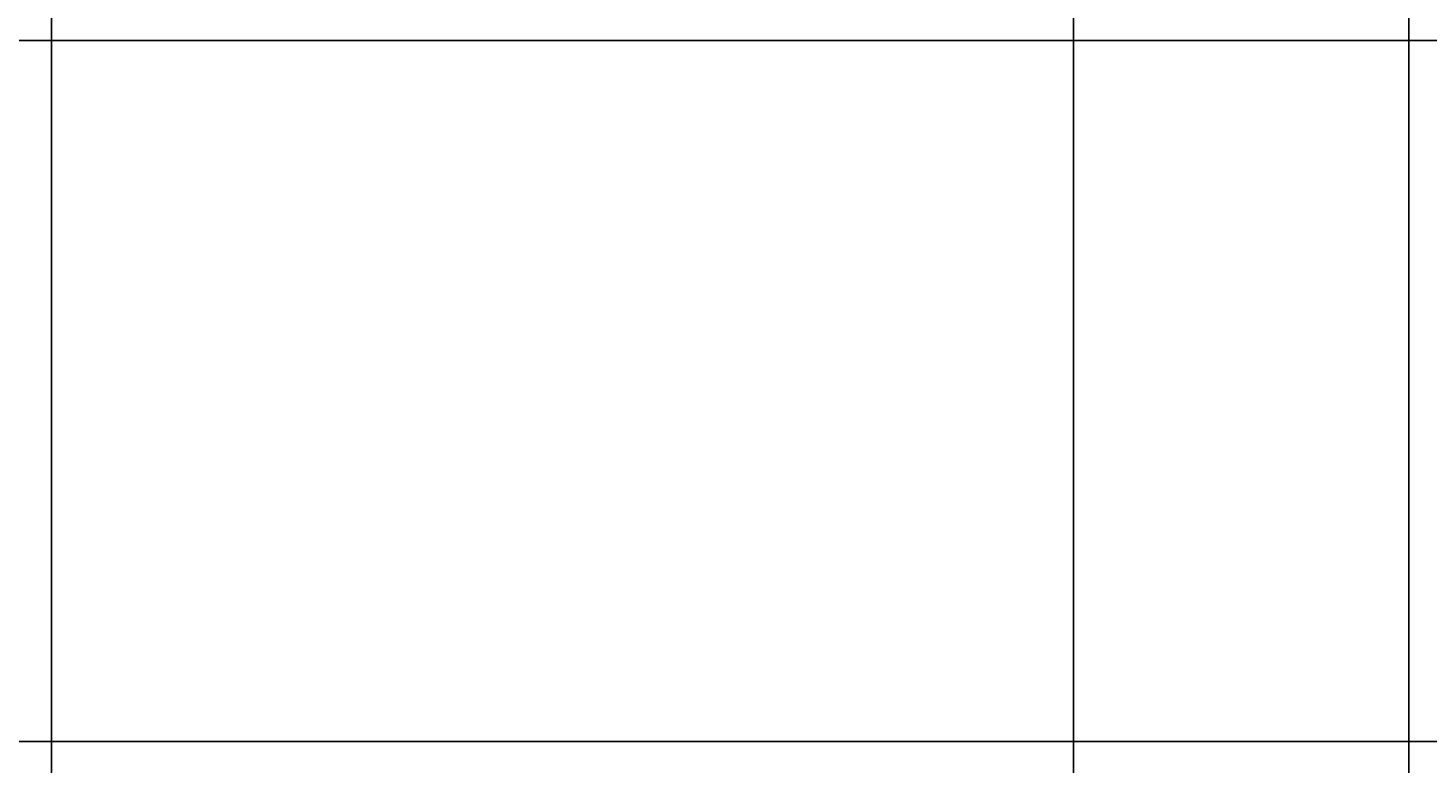
# Model space of a CAD drawing. Units: inches. Extents: x 35362 to 73946, y 43607 to 67532.
# Tile 84 of 134: x 50119 to 51337, y 47689 to 48329. Entities that reach past the tile are written whole.
import ezdxf

# ---------------------------------------------------------------- set-up
doc = ezdxf.new("R2010")
doc.units = ezdxf.units.IN
doc.header["$MEASUREMENT"] = 0
doc.layers.add('A-ANNO-DIMS', color=2, linetype='Continuous', lineweight=18)
doc.styles.get("Standard").update_dxf_attribs({"font": 'arial.ttf'})
doc.dimstyles.get("Standard").update_dxf_attribs({"dimtxt": 0.18, "dimasz": 0.18, "dimexe": 0.18, "dimexo": 0.0625, "dimgap": 0.09, "dimtad": 0, "dimtih": 1, "dimtoh": 1, "dimdec": 4, "dimzin": 0, "dimdsep": 46, "dimtxsty": 'Standard', "dimcen": 0.09, "dimadec": 0, "dimazin": 0, "dimtfac": 1, "dimtdec": 4, "dimtofl": 0, "dimtmove": 0, "dimatfit": 3, "dimfxl": 1, "dimtolj": 1, "dimtzin": 0, "dimarcsym": 0})

# ---------------------------------------------------------------- blocks, each defined once
blk = doc.blocks.new('*D11')
at = {"layer": 'A-ANNO-DIMS', "color": 0, "lineweight": -2, "transparency": 16777216}
for p, q in [((47978.7, 56028.8), (47978.7, 43606.7)), ((53109.8, 56028.8), (53109.8, 43606.7)), ((47978.8, 43606.9), (50543.9, 43606.9)), ((53109.6, 43606.9), (50544.6, 43606.9))]:
    blk.add_line(p, q, dxfattribs=at)
at = {"layer": 'A-ANNO-DIMS', "color": 0, "transparency": 16777216}
for points in [[(47978.8, 43606.9), (47978.8, 43606.8), (47978.7, 43606.9)], [(53109.6, 43606.9), (53109.6, 43606.8), (53109.8, 43606.9)]]:
    blk.add_solid(points, dxfattribs=at)
at = {"layer": 'Defpoints', "color": 0, "transparency": 16777216}
for p in [(47978.7, 56028.8), (53109.8, 56028.8), (53109.8, 43606.9)]:
    blk.add_point(p, dxfattribs=at)
at = {"layer": 'A-ANNO-DIMS', "color": 0, "transparency": 16777216, "insert": (50544.2, 43606.9), "char_height": 0.18, "attachment_point": 5}
blk.add_mtext('\\A1;5131', dxfattribs=at)
blk = doc.blocks.new('*D13')
at = {"layer": 'A-ANNO-DIMS', "color": 0, "lineweight": -2, "transparency": 16777216}
for p, q in [((48373.5, 51694), (48373.5, 43606.7)), ((51029, 51694), (51029, 43606.7)), ((48373.7, 43606.9), (49700.8, 43606.9)), ((51028.9, 43606.9), (49701.7, 43606.9))]:
    blk.add_line(p, q, dxfattribs=at)
at = {"layer": 'A-ANNO-DIMS', "color": 0, "transparency": 16777216}
for points in [[(48373.7, 43606.9), (48373.7, 43606.8), (48373.5, 43606.9)], [(51028.9, 43606.9), (51028.9, 43606.8), (51029, 43606.9)]]:
    blk.add_solid(points, dxfattribs=at)
at = {"layer": 'Defpoints', "color": 0, "transparency": 16777216}
for p in [(48373.5, 51694.1), (51029, 51694.1), (51029, 43606.9)]:
    blk.add_point(p, dxfattribs=at)
at = {"layer": 'A-ANNO-DIMS', "color": 0, "transparency": 16777216, "insert": (49701.3, 43606.9), "char_height": 0.18, "attachment_point": 5}
blk.add_mtext('\\A1;2655.6', dxfattribs=at)
blk = doc.blocks.new('*D17')
at = {"layer": 'A-ANNO-DIMS', "color": 0, "lineweight": -2, "transparency": 16777216}
for p, q in [((49923.3, 61293.2), (49923.3, 43606.7)), ((51913.9, 61293.2), (51913.9, 43606.7)), ((49923.5, 43606.9), (50918.2, 43606.9)), ((51913.8, 43606.9), (50919.1, 43606.9))]:
    blk.add_line(p, q, dxfattribs=at)
at = {"layer": 'A-ANNO-DIMS', "color": 0, "transparency": 16777216}
for points in [[(49923.5, 43606.9), (49923.5, 43606.8), (49923.3, 43606.9)], [(51913.8, 43606.9), (51913.8, 43606.8), (51913.9, 43606.9)]]:
    blk.add_solid(points, dxfattribs=at)
at = {"layer": 'Defpoints', "color": 0, "transparency": 16777216}
for p in [(49923.3, 61293.3), (51913.9, 61293.3), (51913.9, 43606.9)]:
    blk.add_point(p, dxfattribs=at)
at = {"layer": 'A-ANNO-DIMS', "color": 0, "transparency": 16777216, "insert": (50918.6, 43606.9), "char_height": 0.18, "attachment_point": 5}
blk.add_mtext('\\A1;1990.6', dxfattribs=at)
blk = doc.blocks.new('*D67')
at = {"layer": 'A-ANNO-DIMS', "color": 0, "lineweight": -2, "transparency": 16777216}
for p, q in [((56873.5, 53351.5), (35361.8, 53351.5)), ((35361.9, 53351.3), (35361.9, 49400.9)), ((35361.9, 45450.1), (35361.9, 49400.5)), ((53793.6, 45449.9), (35361.8, 45449.9))]:
    blk.add_line(p, q, dxfattribs=at)
at = {"layer": 'A-ANNO-DIMS', "color": 0, "transparency": 16777216}
for points in [[(35361.9, 53351.3), (35362, 53351.3), (35361.9, 53351.5)], [(35361.9, 45450.1), (35362, 45450.1), (35361.9, 45449.9)]]:
    blk.add_solid(points, dxfattribs=at)
at = {"layer": 'Defpoints', "color": 0, "transparency": 16777216}
for p in [(35361.9, 53351.5), (56873.6, 53351.5), (53793.6, 45449.9)]:
    blk.add_point(p, dxfattribs=at)
at = {"layer": 'A-ANNO-DIMS', "color": 0, "transparency": 16777216, "insert": (35361.9, 49400.7), "char_height": 0.18, "attachment_point": 5}
blk.add_mtext('\\A1;7901.6', dxfattribs=at)
blk = doc.blocks.new('*D87')
at = {"layer": 'A-ANNO-DIMS', "color": 0, "lineweight": -2, "transparency": 16777216}
for p, q in [((52362.5, 48318.3), (35361.8, 48318.3)), ((35361.9, 48318.1), (35361.9, 47931.4)), ((35361.9, 47544.3), (35361.9, 47931)), ((52362.5, 47544.1), (35361.8, 47544.1))]:
    blk.add_line(p, q, dxfattribs=at)
at = {"layer": 'A-ANNO-DIMS', "color": 0, "transparency": 16777216}
for points in [[(35361.9, 48318.1), (35362, 48318.1), (35361.9, 48318.3)], [(35361.9, 47544.3), (35362, 47544.3), (35361.9, 47544.1)]]:
    blk.add_solid(points, dxfattribs=at)
at = {"layer": 'Defpoints', "color": 0, "transparency": 16777216}
for p in [(35361.9, 48318.3), (52362.6, 48318.3), (52362.6, 47544.1)]:
    blk.add_point(p, dxfattribs=at)
at = {"layer": 'A-ANNO-DIMS', "color": 0, "transparency": 16777216, "insert": (35361.9, 47931.2), "char_height": 0.18, "attachment_point": 5}
blk.add_mtext('\\A1;774.1', dxfattribs=at)
blk = doc.blocks.new('*D89')
at = {"layer": 'A-ANNO-DIMS', "color": 0, "lineweight": -2, "transparency": 16777216}
for p, q in [((53707.7, 48897.7), (35361.8, 48897.7)), ((35361.9, 48897.6), (35361.9, 48303.2)), ((35361.9, 47708.4), (35361.9, 48302.8)), ((53707.7, 47708.2), (35361.8, 47708.2))]:
    blk.add_line(p, q, dxfattribs=at)
at = {"layer": 'A-ANNO-DIMS', "color": 0, "transparency": 16777216}
for points in [[(35361.9, 48897.6), (35362, 48897.6), (35361.9, 48897.7)], [(35361.9, 47708.4), (35362, 47708.4), (35361.9, 47708.2)]]:
    blk.add_solid(points, dxfattribs=at)
at = {"layer": 'Defpoints', "color": 0, "transparency": 16777216}
for p in [(53707.8, 48897.7), (35361.9, 47708.2), (53707.8, 47708.2)]:
    blk.add_point(p, dxfattribs=at)
at = {"layer": 'A-ANNO-DIMS', "color": 0, "transparency": 16777216, "insert": (35361.9, 48303), "char_height": 0.18, "attachment_point": 5}
blk.add_mtext('\\A1;1189.5', dxfattribs=at)
blk = doc.blocks.new('*D107')
at = {"layer": 'A-ANNO-DIMS', "color": 0, "lineweight": -2, "transparency": 16777216}
for p, q in [((50139.6, 59850), (50139.6, 43606.7)), ((51320.8, 59850), (51320.8, 43606.7)), ((50139.7, 43606.9), (50729.7, 43606.9)), ((51320.6, 43606.9), (50730.6, 43606.9))]:
    blk.add_line(p, q, dxfattribs=at)
at = {"layer": 'A-ANNO-DIMS', "color": 0, "transparency": 16777216}
for points in [[(50139.7, 43606.9), (50139.7, 43606.8), (50139.6, 43606.9)], [(51320.6, 43606.9), (51320.6, 43606.8), (51320.8, 43606.9)]]:
    blk.add_solid(points, dxfattribs=at)
at = {"layer": 'Defpoints', "color": 0, "transparency": 16777216}
for p in [(50139.6, 59850.1), (51320.8, 59850.1), (51320.8, 43606.9)]:
    blk.add_point(p, dxfattribs=at)
at = {"layer": 'A-ANNO-DIMS', "color": 0, "transparency": 16777216, "insert": (50730.2, 43606.9), "char_height": 0.18, "attachment_point": 5}
blk.add_mtext('\\A1;1181.3', dxfattribs=at)

msp = doc.modelspace()

# ---------------------------------------------------------------- dimensions: what is measured, and where the dimension line sits
at = {"layer": 'A-ANNO-DIMS'}
for base, p1, p2, override, picture, middle in [((51913.931, 43606.859), (49923.307, 61293.286), (51913.931, 61293.286), {"dimdec": 1, "dimlfac": 1, "dimrnd": 0, "dimzin": 0, "dimdsep": 46, "dimlunit": 2}, '*D17', (50918.619, 43606.859)), ((51320.8133, 43606.859), (50139.5627, 59850.0769), (51320.8133, 59850.0769), {"dimdec": 1, "dimlfac": 1, "dimrnd": 0, "dimzin": 0, "dimdsep": 46, "dimlunit": 2}, '*D107', (50730.188, 43606.859)), ((53109.76, 43606.859), (47978.665, 56028.836), (53109.76, 56028.836), {"dimdec": 0, "dimlfac": 1, "dimrnd": 0, "dimzin": 0, "dimdsep": 46, "dimlunit": 2}, '*D11', (50544.212, 43606.859)), ((51029.043, 43606.859), (48373.492, 51694.087), (51029.043, 51694.087), {"dimdec": 1, "dimlfac": 1, "dimrnd": 0, "dimzin": 0, "dimdsep": 46, "dimlunit": 2}, '*D13', (49701.267, 43606.859))]:
    dim = msp.add_linear_dim(base=base, p1=p1, p2=p2, dimstyle='Standard', override=override, dxfattribs=at)
    dim.commit()
    dim.dimension.update_dxf_attribs({"geometry": picture, "text_midpoint": middle})
for base, p1, p2, picture, middle in [((35361.949, 53351.529), (53793.638, 45449.894), (56873.602, 53351.529), '*D67', (35361.949, 49400.712)), ((35361.949, 47708.216), (53707.781, 48897.738), (53707.781, 47708.216), '*D89', (35361.949, 48302.977)), ((35361.949, 48318.269), (52362.557, 47544.134), (52362.557, 48318.269), '*D87', (35361.949, 47931.201))]:
    dim = msp.add_linear_dim(base=base, p1=p1, p2=p2, angle=90, dimstyle='Standard', override={"dimdec": 1, "dimlfac": 1, "dimrnd": 0, "dimzin": 0, "dimdsep": 46, "dimlunit": 2}, dxfattribs=at)
    dim.commit()
    dim.dimension.update_dxf_attribs({"geometry": picture, "text_midpoint": middle})

doc.saveas('drawing.dxf')
